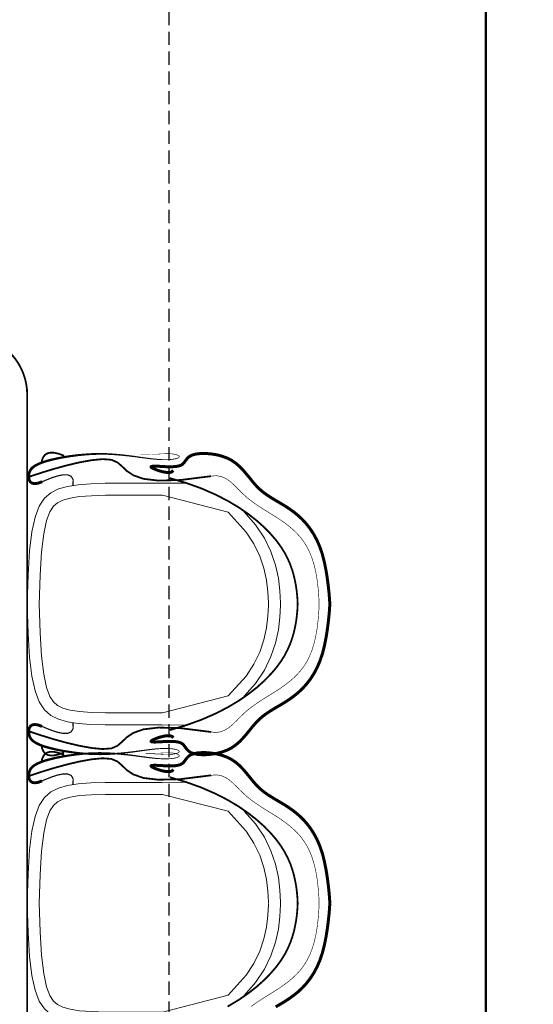
# Model space of a CAD drawing. Units: inches. Extents: x 513 to 1142, y 396 to 927.
# Tile 18 of 31: x 818 to 838, y 728 to 766. Entities that reach past the tile are written whole.
import ezdxf

# ---------------------------------------------------------------- set-up
doc = ezdxf.new("R2010")
doc.units = ezdxf.units.IN
doc.header["$MEASUREMENT"] = 0
doc.linetypes.add('DASHED', pattern=[0.75, 0.5, -0.25])
for name, color, linetype, lineweight in [('A-ANNO-DIMS', 2, 'DASHED', 18), ('A-WALL', 7, 'Continuous', 50), ('furniture', 92, 'Continuous', 18)]:
    doc.layers.add(name, color=color, linetype=linetype, lineweight=lineweight)
doc.styles.get("Standard").update_dxf_attribs({"font": 'arial.ttf'})
doc.dimstyles.get("Standard").update_dxf_attribs({"dimtxt": 4, "dimasz": 0.18, "dimexe": 0.18, "dimexo": 0.0625, "dimgap": 0.09, "dimtad": 0, "dimtih": 1, "dimtoh": 1, "dimdec": 0, "dimrnd": 6, "dimzin": 0, "dimdsep": 46, "dimlunit": 3, "dimtxsty": 'Standard', "dimcen": 0.09, "dimadec": 0, "dimazin": 0, "dimtfac": 1, "dimtdec": 0, "dimtofl": 0, "dimtmove": 0, "dimatfit": 3, "dimfxl": 1, "dimtolj": 1, "dimtzin": 0, "dimarcsym": 0})

# ---------------------------------------------------------------- blocks, each defined once
blk = doc.blocks.new('ОГ55_на6персон_стол1400х900')
at = {"const_width": 3}
blk.add_lwpolyline([(-600, 279.3), (600, 279.3, -0.414214), (700, 179.3), (700, -520.7, -0.414214), (600, -620.7), (-600, -620.7, -0.414214), (-700, -520.7), (-700, 179.3, -0.414214)], format="xyb", close=True, dxfattribs=at)
for points in [[(-452.3, -886.8), (-451.9, -846.4), (-451.9, -810.6), (-452, -778.9), (-451.9, -751.1), (-451.2, -726.9), (-449.6, -706), (-446.8, -688.1), (-442.5, -672.9), (-436.1, -660), (-426.8, -649.4), (-413.5, -640.7), (-395.1, -633.9), (-370.6, -628.7), (-339, -624.8), (-299.1, -622.2), (-250, -620.7)], [(-47.7, -886.8), (-48.1, -846.4), (-48.1, -810.6), (-48, -778.9), (-48.1, -751.1), (-48.8, -726.9), (-50.4, -706), (-53.2, -688.1), (-57.5, -672.9), (-63.9, -660), (-73.2, -649.4), (-86.5, -640.7), (-104.9, -633.9), (-129.4, -628.7), (-161, -624.8), (-200.9, -622.2), (-250, -620.7)], [(47.7, -886.8), (48.1, -846.4), (48.1, -810.6), (48, -778.9), (48.1, -751.1), (48.8, -726.9), (50.4, -706), (53.2, -688.1), (57.5, -672.9), (63.9, -660), (73.2, -649.4), (86.5, -640.7), (104.9, -633.9), (129.4, -628.7), (161, -624.8), (200.9, -622.2), (250, -620.7)], [(452.3, -886.8), (451.9, -846.4), (451.9, -810.6), (452, -778.9), (451.9, -751.1), (451.2, -726.9), (449.6, -706), (446.8, -688.1), (442.5, -672.9), (436.1, -660), (426.8, -649.4), (413.5, -640.7), (395.1, -633.9), (370.6, -628.7), (339, -624.8), (299.1, -622.2), (250, -620.7)], [(-403.6, -956.4), (-431.9, -846.6), (-431.9, -810.5), (-432, -778.9), (-431.9, -751.4), (-431.2, -728), (-429.8, -708.3), (-427.3, -692.4), (-423.8, -680.1), (-419.4, -671.3), (-413.6, -664.7), (-404.4, -658.7), (-389.5, -653.1), (-367.3, -648.4), (-337.1, -644.8), (-298.1, -642.2), (-249.4, -640.7)], [(-96.4, -956.4), (-68.1, -846.6), (-68.1, -810.5), (-68, -778.9), (-68.1, -751.4), (-68.8, -728), (-70.2, -708.3), (-72.7, -692.4), (-76.2, -680.1), (-80.6, -671.3), (-86.4, -664.7), (-95.6, -658.7), (-110.5, -653.1), (-132.7, -648.4), (-162.9, -644.8), (-201.9, -642.2), (-250.6, -640.7)], [(96.4, -956.4), (68.1, -846.6), (68.1, -810.5), (68, -778.9), (68.1, -751.4), (68.8, -728), (70.2, -708.3), (72.7, -692.4), (76.2, -680.1), (80.6, -671.3), (86.4, -664.7), (95.6, -658.7), (110.5, -653.1), (132.7, -648.4), (162.9, -644.8), (201.9, -642.2), (250.6, -640.7)], [(403.6, -956.4), (431.9, -846.6), (431.9, -810.5), (432, -778.9), (431.9, -751.4), (431.2, -728), (429.8, -708.3), (427.3, -692.4), (423.8, -680.1), (419.4, -671.3), (413.6, -664.7), (404.4, -658.7), (389.5, -653.1), (367.3, -648.4), (337.1, -644.8), (298.1, -642.2), (249.4, -640.7)], [(-403.6, -956.4), (-370.3, -986.3), (-350.5, -999.5), (-330.2, -1009.3), (-309.8, -1016.2), (-289.8, -1020.6), (-270.4, -1023), (-252.1, -1023.8), (-250.4, -1023.8)], [(-96.4, -956.4), (-129.7, -986.3), (-149.5, -999.5), (-169.8, -1009.3), (-190.2, -1016.2), (-210.2, -1020.6), (-229.6, -1023), (-247.9, -1023.8), (-249.6, -1023.8)], [(96.4, -956.4), (129.7, -986.3), (149.5, -999.5), (169.8, -1009.3), (190.2, -1016.2), (210.2, -1020.6), (229.6, -1023), (247.9, -1023.8), (249.6, -1023.8)], [(403.6, -956.4), (370.3, -986.3), (350.5, -999.5), (330.2, -1009.3), (309.8, -1016.2), (289.8, -1020.6), (270.4, -1023), (252.1, -1023.8), (250.4, -1023.8)], [(-404, -983), (-382.6, -1002.1), (-360.4, -1016.9), (-337.8, -1027.9), (-315.2, -1035.5), (-293.1, -1040.4), (-272, -1043), (-252.3, -1043.8), (-250, -1043.8)], [(-96, -983), (-117.4, -1002.1), (-139.6, -1016.9), (-162.2, -1027.9), (-184.8, -1035.5), (-206.9, -1040.4), (-228, -1043), (-247.7, -1043.8), (-250, -1043.8)], [(96, -983), (117.4, -1002.1), (139.6, -1016.9), (162.2, -1027.9), (184.8, -1035.5), (206.9, -1040.4), (228, -1043), (247.7, -1043.8), (250, -1043.8)], [(404, -983), (382.6, -1002.1), (360.4, -1016.9), (337.8, -1027.9), (315.2, -1035.5), (293.1, -1040.4), (272, -1043), (252.3, -1043.8), (250, -1043.8)]]:
    blk.add_lwpolyline(points)
for points in [[(-45.5, -645.6, 5, 4.91, 0), (-48, -638.8, 4.91, 4.84, 0), (-48.7, -633.5, 4.84, 4.78, 0), (-48.1, -629.4, 4.78, 4.74, 0), (-46.3, -626.5, 4.74, 4.7, 0), (-43.7, -624.6, 4.7, 4.65, 0), (-40.6, -623.5, 4.65, 4.61, 0), (-37.1, -623.2, 4.61, 4.56, 0), (-33.5, -623.5, 4.56, 4.52, 0), (-30.2, -624.2, 4.52, 4.47, 0), (-27.1, -625.5, 4.47, 4.43, 0), (-24.1, -627.4, 4.43, 4.38, 0), (-21.3, -630.2, 4.38, 4.32, 0), (-18.7, -633.9, 4.32, 4.25, 0), (-16.2, -638.6, 4.25, 4.17, 0), (-13.7, -644.5, 4.17, 4.07, 0), (-11.3, -651.7, 4.07, 3.95, 0), (-9, -660.3, 3.95, 3.82, 0), (-6.7, -670, 3.82, 3.68, 0), (-4.6, -680.8, 3.68, 3.53, 0), (-2.8, -692.3, 3.53, 3.37, 0), (-1.2, -704.4, 3.37, 3.21, 0), (0, -716.9, 3.21, 3.05, 0), (0.8, -729.5, 3.05, 2.88, 0), (1.1, -742.1, 2.88, 2.72, 0), (0.9, -754.5, 2.72, 2.57, 0), (0.2, -766.5, 2.57, 2.41, 0), (-0.8, -778.1, 2.41, 2.27, 0), (-2, -789.2, 2.27, 2.13, 0), (-3.3, -799.7, 2.13, 2, 0), (-4.7, -809.6, 2, 1.88, 0), (-5.9, -818.7, 1.88, 1.78, 0), (-7, -827, 1.78, 1.68, 0), (-7.8, -834.4, 1.68, 1.59, 0), (-8.3, -841, 1.59, 1.52, 0), (-8.6, -846.8, 1.52, 1.45, 0), (-8.7, -851.9, 1.45, 1.4, 0), (-8.6, -856.3, 1.4, 1.35, 0), (-8.4, -860.1, 1.35, 1.3, 0), (-8, -863.3, 1.3, 1.27, 0), (-7.6, -866, 1.27, 1.24, 0), (-7.2, -868.3, 1.24, 1.21, 0), (-6.7, -870.2, 1.21, 1.19, 0), (-6.2, -871.7, 1.19, 1.18, 0), (-5.7, -872.9, 1.18, 1.16, 0), (-5.2, -873.7, 1.16, 1.15, 0), (-4.7, -874.3, 1.15, 1.14, 0), (-4.2, -874.6, 1.14, 1.14, 0), (-3.7, -874.7, 1.14, 1.13, 0), (-3.2, -874.6, 1.13, 1.12, 0), (-2.7, -874.3, 1.12, 1.12, 0), (-2.2, -873.9, 1.12, 1.11, 0), (-1.7, -873.3, 1.11, 1.09, 0), (-1.3, -872.5, 1.09, 1.08, 0), (-0.9, -871.6, 1.08, 1.07, 0), (-0.5, -870.5, 1.07, 1.05, 0), (-0.1, -869.2, 1.05, 1.03, 0), (0.3, -867.9, 1.03, 1.01, 0), (0.6, -866.3, 1.01, 0.986, 0), (0.9, -864.5, 0.986, 0.959, 0), (1.1, -862.4, 0.959, 0.926, 0), (1.3, -859.9, 0.926, 0.889, 0), (1.4, -857, 0.889, 0.846, 0), (1.4, -853.7, 0.846, 0.796, 0), (1.3, -849.8, 0.796, 0.738, 0), (1.1, -845.4, 0.738, 0.672, 0), (0.8, -840.3, 0.672, 0.595, 0), (0.6, -834.3, 0.595, 0.506, 0), (0.3, -827.5, 0.506, 0.404, 0), (0.1, -819.6, 0.404, 0.286, 0), (-0.1, -810.5, 0.286, 0.152, 0), (-0.1, -800.2, 0.152, 0, 0), (0, -788.5, 0, 0, 0)], [(45.5, -645.6, 5, 4.91, 0), (48, -638.8, 4.91, 4.84, 0), (48.7, -633.5, 4.84, 4.78, 0), (48.1, -629.4, 4.78, 4.74, 0), (46.3, -626.5, 4.74, 4.7, 0), (43.7, -624.6, 4.7, 4.65, 0), (40.6, -623.5, 4.65, 4.61, 0), (37.1, -623.2, 4.61, 4.56, 0), (33.5, -623.5, 4.56, 4.52, 0), (30.2, -624.2, 4.52, 4.47, 0), (27.1, -625.5, 4.47, 4.43, 0), (24.1, -627.4, 4.43, 4.38, 0), (21.3, -630.2, 4.38, 4.32, 0), (18.7, -633.9, 4.32, 4.25, 0), (16.2, -638.6, 4.25, 4.17, 0), (13.7, -644.5, 4.17, 4.07, 0), (11.3, -651.7, 4.07, 3.95, 0), (9, -660.3, 3.95, 3.82, 0), (6.7, -670, 3.82, 3.68, 0), (4.6, -680.8, 3.68, 3.53, 0), (2.8, -692.3, 3.53, 3.37, 0), (1.2, -704.4, 3.37, 3.21, 0), (0, -716.9, 3.21, 3.05, 0), (-0.8, -729.5, 3.05, 2.88, 0), (-1.1, -742.1, 2.88, 2.72, 0), (-0.9, -754.5, 2.72, 2.57, 0), (-0.2, -766.5, 2.57, 2.41, 0), (0.8, -778.1, 2.41, 2.27, 0), (2, -789.2, 2.27, 2.13, 0), (3.3, -799.7, 2.13, 2, 0), (4.7, -809.6, 2, 1.88, 0), (5.9, -818.7, 1.88, 1.78, 0), (7, -827, 1.78, 1.68, 0), (7.8, -834.4, 1.68, 1.59, 0), (8.3, -841, 1.59, 1.52, 0), (8.6, -846.8, 1.52, 1.45, 0), (8.7, -851.9, 1.45, 1.4, 0), (8.6, -856.3, 1.4, 1.35, 0), (8.4, -860.1, 1.35, 1.3, 0), (8, -863.3, 1.3, 1.27, 0), (7.6, -866, 1.27, 1.24, 0), (7.2, -868.3, 1.24, 1.21, 0), (6.7, -870.2, 1.21, 1.19, 0), (6.2, -871.7, 1.19, 1.18, 0), (5.7, -872.9, 1.18, 1.16, 0), (5.2, -873.7, 1.16, 1.15, 0), (4.7, -874.3, 1.15, 1.14, 0), (4.2, -874.6, 1.14, 1.14, 0), (3.7, -874.7, 1.14, 1.13, 0), (3.2, -874.6, 1.13, 1.12, 0), (2.7, -874.3, 1.12, 1.12, 0), (2.2, -873.9, 1.12, 1.11, 0), (1.7, -873.3, 1.11, 1.09, 0), (1.3, -872.5, 1.09, 1.08, 0), (0.9, -871.6, 1.08, 1.07, 0), (0.5, -870.5, 1.07, 1.05, 0), (0.1, -869.2, 1.05, 1.03, 0), (-0.3, -867.9, 1.03, 1.01, 0), (-0.6, -866.3, 1.01, 0.986, 0), (-0.9, -864.5, 0.986, 0.959, 0), (-1.1, -862.4, 0.959, 0.926, 0), (-1.3, -859.9, 0.926, 0.889, 0), (-1.4, -857, 0.889, 0.846, 0), (-1.4, -853.7, 0.846, 0.796, 0), (-1.3, -849.8, 0.796, 0.738, 0), (-1.1, -845.4, 0.738, 0.672, 0), (-0.8, -840.3, 0.672, 0.595, 0), (-0.6, -834.3, 0.595, 0.506, 0), (-0.3, -827.5, 0.506, 0.404, 0), (-0.1, -819.6, 0.404, 0.286, 0), (0.1, -810.5, 0.286, 0.152, 0), (0.1, -800.2, 0.152, 0, 0), (0, -788.5, 0, 0, 0)], [(454.5, -645.6, 5, 4.91, 0), (452, -638.8, 4.91, 4.84, 0), (451.3, -633.5, 4.84, 4.78, 0), (451.9, -629.4, 4.78, 4.74, 0), (453.7, -626.5, 4.74, 4.7, 0), (456.3, -624.6, 4.7, 4.65, 0), (459.4, -623.5, 4.65, 4.61, 0), (462.9, -623.2, 4.61, 4.56, 0), (466.5, -623.5, 4.56, 4.52, 0), (469.8, -624.2, 4.52, 4.47, 0), (472.9, -625.5, 4.47, 4.43, 0), (475.9, -627.4, 4.43, 4.38, 0), (478.7, -630.2, 4.38, 4.32, 0), (481.3, -633.9, 4.32, 4.25, 0), (483.8, -638.6, 4.25, 4.17, 0), (486.3, -644.5, 4.17, 4.07, 0), (488.7, -651.7, 4.07, 3.95, 0), (491, -660.3, 3.95, 3.82, 0), (493.3, -670, 3.82, 3.68, 0), (495.4, -680.8, 3.68, 3.53, 0), (497.2, -692.3, 3.53, 3.37, 0), (498.8, -704.4, 3.37, 3.21, 0), (500, -716.9, 3.21, 3.05, 0), (500.8, -729.5, 3.05, 2.88, 0), (501.1, -742.1, 2.88, 2.72, 0), (500.9, -754.5, 2.72, 2.57, 0), (500.2, -766.5, 2.57, 2.41, 0), (499.2, -778.1, 2.41, 2.27, 0), (498, -789.2, 2.27, 2.13, 0), (496.7, -799.7, 2.13, 2, 0), (495.3, -809.6, 2, 1.88, 0), (494.1, -818.7, 1.88, 1.78, 0), (493, -827, 1.78, 1.68, 0), (492.2, -834.4, 1.68, 1.59, 0), (491.7, -841, 1.59, 1.52, 0), (491.4, -846.8, 1.52, 1.45, 0), (491.3, -851.9, 1.45, 1.4, 0), (491.4, -856.3, 1.4, 1.35, 0), (491.6, -860.1, 1.35, 1.3, 0), (492, -863.3, 1.3, 1.27, 0), (492.4, -866, 1.27, 1.24, 0), (492.8, -868.3, 1.24, 1.21, 0), (493.3, -870.2, 1.21, 1.19, 0), (493.8, -871.7, 1.19, 1.18, 0), (494.3, -872.9, 1.18, 1.16, 0), (494.8, -873.7, 1.16, 1.15, 0), (495.3, -874.3, 1.15, 1.14, 0), (495.8, -874.6, 1.14, 1.14, 0), (496.3, -874.7, 1.14, 1.13, 0), (496.8, -874.6, 1.13, 1.12, 0), (497.3, -874.3, 1.12, 1.12, 0), (497.8, -873.9, 1.12, 1.11, 0), (498.3, -873.3, 1.11, 1.09, 0), (498.7, -872.5, 1.09, 1.08, 0), (499.1, -871.6, 1.08, 1.07, 0), (499.5, -870.5, 1.07, 1.05, 0), (499.9, -869.2, 1.05, 1.03, 0), (500.3, -867.9, 1.03, 1.01, 0), (500.6, -866.3, 1.01, 0.986, 0), (500.9, -864.5, 0.986, 0.959, 0), (501.1, -862.4, 0.959, 0.926, 0), (501.3, -859.9, 0.926, 0.889, 0), (501.4, -857, 0.889, 0.846, 0), (501.4, -853.7, 0.846, 0.796, 0), (501.3, -849.8, 0.796, 0.738, 0), (501.1, -845.4, 0.738, 0.672, 0), (500.8, -840.3, 0.672, 0.595, 0), (500.6, -834.3, 0.595, 0.506, 0), (500.3, -827.5, 0.506, 0.404, 0), (500.1, -819.6, 0.404, 0.286, 0), (499.9, -810.5, 0.286, 0.152, 0), (499.9, -800.2, 0.152, 0, 0), (500, -788.5, 0, 0, 0)]]:
    blk.add_lwpolyline(points, format="xyseb")
for points, const_width in [([(-36.2, -927.9), (-42.6, -876.9), (-43.6, -840.1), (-40.6, -814.7), (-34.7, -798), (-27.4, -787), (-19.8, -779.2), (-13.2, -771.5), (-8.8, -761.4), (-7.7, -746.6), (-9.5, -728.1), (-13.3, -707.3), (-18.4, -685.8), (-24.1, -665.1), (-29.7, -646.8), (-34.4, -632.3), (-37.5, -623.2)], 3), ([(36.2, -927.9), (42.6, -876.9), (43.6, -840.1), (40.6, -814.7), (34.7, -798), (27.4, -787), (19.8, -779.2), (13.2, -771.5), (8.8, -761.4), (7.7, -746.6), (9.5, -728.1), (13.3, -707.3), (18.4, -685.8), (24.1, -665.1), (29.7, -646.8), (34.4, -632.3), (37.5, -623.2)], 3), ([(463.8, -927.9), (457.4, -876.9), (456.4, -840.1), (459.4, -814.7), (465.3, -798), (472.6, -787), (480.2, -779.2), (486.8, -771.5), (491.2, -761.4), (492.3, -746.6), (490.5, -728.1), (486.7, -707.3), (481.6, -685.8), (475.9, -665.1), (470.3, -646.8), (465.6, -632.3), (462.5, -623.2)], 3), ([(-45.5, -645.6), (-42.2, -653.4), (-38.7, -662.3), (-35.7, -671.7), (-33.9, -680.7), (-34, -688.5), (-36.5, -694.3), (-42.2, -697.5), (-51.8, -697.1)], 2), ([(-2, -682.4), (1.3, -673.2), (3, -665.5), (3.1, -659.2), (1.9, -654.2), (-0.6, -650.4), (-4.2, -647.6), (-8.8, -645.6), (-14.3, -644.5)], 3), ([(2, -682.4), (-1.3, -673.2), (-3, -665.5), (-3.1, -659.2), (-1.9, -654.2), (0.6, -650.4), (4.2, -647.6), (8.8, -645.6), (14.3, -644.5)], 3), ([(45.5, -645.6), (42.2, -653.4), (38.7, -662.3), (35.7, -671.7), (33.9, -680.7), (34, -688.5), (36.5, -694.3), (42.2, -697.5), (51.8, -697.1)], 2), ([(454.5, -645.6), (457.8, -653.4), (461.3, -662.3), (464.3, -671.7), (466.1, -680.7), (466, -688.5), (463.5, -694.3), (457.8, -697.5), (448.2, -697.1)], 2), ([(498, -682.4), (501.3, -673.2), (503, -665.5), (503.1, -659.2), (501.9, -654.2), (499.4, -650.4), (495.8, -647.6), (491.2, -645.6), (485.7, -644.5)], 3), ([(-423.2, -1035.9), (-418.9, -1043.3), (-414.4, -1050.8), (-409.5, -1058.3), (-404.2, -1065.7), (-398.3, -1073), (-391.7, -1080.1), (-384.3, -1086.9), (-376.1, -1093.3), (-366.9, -1099.3), (-356.7, -1104.8), (-345.4, -1109.7), (-333, -1113.9), (-319.5, -1117.3), (-305.4, -1120.1), (-291.5, -1122.3), (-278.6, -1123.9), (-267.2, -1125.1), (-258.2, -1125.8), (-252.2, -1126.2), (-250, -1126.3)], 5), ([(-26.6, -864.8), (-28.8, -862.7), (-29.9, -859.6), (-30.1, -855.5), (-29.6, -851), (-28.6, -846.2), (-27.3, -841.5), (-25.8, -837.1), (-24.3, -833.4), (-23, -830.6), (-22, -828.7), (-21.1, -827.8), (-20.4, -827.7), (-19.9, -828.6), (-19.6, -830.5), (-19.4, -833.2), (-19.5, -836.7), (-19.7, -841.2), (-20, -846.2), (-20.3, -851.7), (-20.4, -857.3), (-20.4, -862.9), (-20.1, -868.2), (-19.4, -872.9), (-18.2, -876.8), (-16.5, -879.9), (-14.3, -882.2), (-11.8, -884.1), (-9.2, -886), (-6.6, -888), (-4.1, -890.6), (-1.9, -894), (-0.2, -898.6), (1.1, -904.5), (1.7, -911.6), (1.7, -919.5), (1, -928), (-0.4, -936.8), (-2.6, -945.6), (-5.7, -954.1), (-9.6, -962), (-14.5, -969.1), (-20, -975.5), (-26.1, -981.4), (-32.5, -986.9), (-39.1, -992.3), (-45.7, -997.6), (-51.9, -1003), (-57.8, -1008.8), (-63.1, -1015.1), (-67.9, -1021.7), (-72.4, -1028.7), (-76.8, -1035.9), (-81.1, -1043.3), (-85.6, -1050.8), (-90.5, -1058.3), (-95.8, -1065.7), (-101.7, -1073), (-108.3, -1080.1), (-115.7, -1086.9), (-123.9, -1093.3), (-133.1, -1099.3), (-143.3, -1104.8), (-154.6, -1109.7), (-167, -1113.9), (-180.5, -1117.3), (-194.6, -1120.1), (-208.5, -1122.3), (-221.4, -1123.9), (-232.8, -1125.1), (-241.8, -1125.8), (-247.8, -1126.2), (-250, -1126.3)], 5), ([(26.6, -864.8), (28.8, -862.7), (29.9, -859.6), (30.1, -855.5), (29.6, -851), (28.6, -846.2), (27.3, -841.5), (25.8, -837.1), (24.3, -833.4), (23, -830.6), (22, -828.7), (21.1, -827.8), (20.4, -827.7), (19.9, -828.6), (19.6, -830.5), (19.4, -833.2), (19.5, -836.7), (19.7, -841.2), (20, -846.2), (20.3, -851.7), (20.4, -857.3), (20.4, -862.9), (20.1, -868.2), (19.4, -872.9), (18.2, -876.8), (16.5, -879.9), (14.3, -882.2), (11.8, -884.1), (9.2, -886), (6.6, -888), (4.1, -890.6), (1.9, -894), (0.2, -898.6), (-1.1, -904.5), (-1.7, -911.6), (-1.7, -919.5), (-1, -928), (0.4, -936.8), (2.6, -945.6), (5.7, -954.1), (9.6, -962), (14.5, -969.1), (20, -975.5), (26.1, -981.4), (32.5, -986.9), (39.1, -992.3), (45.7, -997.6), (51.9, -1003), (57.8, -1008.8), (63.1, -1015.1), (67.9, -1021.7), (72.4, -1028.7), (76.8, -1035.9), (81.1, -1043.3), (85.6, -1050.8), (90.5, -1058.3), (95.8, -1065.7), (101.7, -1073), (108.3, -1080.1), (115.7, -1086.9), (123.9, -1093.3), (133.1, -1099.3), (143.3, -1104.8), (154.6, -1109.7), (167, -1113.9), (180.5, -1117.3), (194.6, -1120.1), (208.5, -1122.3), (221.4, -1123.9), (232.8, -1125.1), (241.8, -1125.8), (247.8, -1126.2), (250, -1126.3)], 5), ([(473.4, -864.8), (471.2, -862.7), (470.1, -859.6), (469.9, -855.5), (470.4, -851), (471.4, -846.2), (472.7, -841.5), (474.2, -837.1), (475.7, -833.4), (477, -830.6), (478, -828.7), (478.9, -827.8), (479.6, -827.7), (480.1, -828.6), (480.4, -830.5), (480.6, -833.2), (480.5, -836.7), (480.3, -841.2), (480, -846.2), (479.7, -851.7), (479.6, -857.3), (479.6, -862.9), (479.9, -868.2), (480.6, -872.9), (481.8, -876.8), (483.5, -879.9), (485.7, -882.2), (488.2, -884.1), (490.8, -886), (493.4, -888), (495.9, -890.6), (498.1, -894), (499.8, -898.6), (501.1, -904.5), (501.7, -911.6), (501.7, -919.5), (501, -928), (499.6, -936.8), (497.4, -945.6), (494.3, -954.1), (490.4, -962), (485.5, -969.1), (480, -975.5), (473.9, -981.4), (467.5, -986.9), (460.9, -992.3), (454.3, -997.6), (448.1, -1003), (442.2, -1008.8), (436.9, -1015.1), (432.1, -1021.7), (427.6, -1028.7), (423.2, -1035.9), (418.9, -1043.3), (414.4, -1050.8), (409.5, -1058.3), (404.2, -1065.7), (398.3, -1073), (391.7, -1080.1), (384.3, -1086.9), (376.1, -1093.3), (366.9, -1099.3), (356.7, -1104.8), (345.4, -1109.7), (333, -1113.9), (319.5, -1117.3), (305.4, -1120.1), (291.5, -1122.3), (278.6, -1123.9), (267.2, -1125.1), (258.2, -1125.8), (252.2, -1126.2), (250, -1126.3)], 5), ([(-422.7, -955.5), (-411.8, -973.8), (-400.6, -990), (-389.4, -1004.3), (-378.2, -1016.8), (-367.2, -1027.5), (-356.5, -1036.7), (-346, -1044.4), (-335.8, -1050.8), (-325.7, -1056), (-315.9, -1060.3), (-306.4, -1063.6), (-297, -1066.3), (-287.9, -1068.3), (-279.3, -1069.9), (-271.3, -1071), (-264.3, -1071.7), (-258.4, -1072.2), (-253.9, -1072.4), (-251, -1072.5), (-250, -1072.5)], 3), ([(-39.4, -859), (-47.7, -886.8), (-56.8, -912.1), (-66.8, -934.9), (-77.3, -955.5), (-88.2, -973.8), (-99.4, -990), (-110.6, -1004.3), (-121.8, -1016.8), (-132.8, -1027.5), (-143.5, -1036.7), (-154, -1044.4), (-164.2, -1050.8), (-174.3, -1056), (-184.1, -1060.3), (-193.6, -1063.6), (-203, -1066.3), (-212.1, -1068.3), (-220.7, -1069.9), (-228.7, -1071), (-235.7, -1071.7), (-241.6, -1072.2), (-246.1, -1072.4), (-249, -1072.5), (-250, -1072.5)], 3), ([(39.4, -859), (47.7, -886.8), (56.8, -912.1), (66.8, -934.9), (77.3, -955.5), (88.2, -973.8), (99.4, -990), (110.6, -1004.3), (121.8, -1016.8), (132.8, -1027.5), (143.5, -1036.7), (154, -1044.4), (164.2, -1050.8), (174.3, -1056), (184.1, -1060.3), (193.6, -1063.6), (203, -1066.3), (212.1, -1068.3), (220.7, -1069.9), (228.7, -1071), (235.7, -1071.7), (241.6, -1072.2), (246.1, -1072.4), (249, -1072.5), (250, -1072.5)], 3), ([(460.6, -859), (452.3, -886.8), (443.2, -912.1), (433.2, -934.9), (422.7, -955.5), (411.8, -973.8), (400.6, -990), (389.4, -1004.3), (378.2, -1016.8), (367.2, -1027.5), (356.5, -1036.7), (346, -1044.4), (335.8, -1050.8), (325.7, -1056), (315.9, -1060.3), (306.4, -1063.6), (297, -1066.3), (287.9, -1068.3), (279.3, -1069.9), (271.3, -1071), (264.3, -1071.7), (258.4, -1072.2), (253.9, -1072.4), (251, -1072.5), (250, -1072.5)], 3), ([(-422.8, -994.6), (-417.9, -1001.3), (-413.3, -1008.1), (-408.8, -1015), (-404.4, -1022.1), (-400, -1029.2), (-395.5, -1036.4), (-390.8, -1043.6), (-385.8, -1050.7), (-380.5, -1057.7), (-374.7, -1064.5), (-368.5, -1071), (-361.7, -1077.1), (-354.1, -1082.8), (-345.9, -1088), (-336.7, -1092.6), (-326.7, -1096.6), (-315.5, -1100), (-303.3, -1102.9), (-289.8, -1105.2), (-274.9, -1106.9), (-258.6, -1108.1), (-250, -1108.4)], 1), ([(-36.2, -927.9), (-35.4, -936.5), (-36.6, -944.3), (-39.5, -951.4), (-43.7, -958), (-48.9, -964.1), (-54.7, -970.1), (-60.7, -976), (-66.6, -982), (-72.1, -988.2), (-77.2, -994.6), (-82.1, -1001.3), (-86.7, -1008.1), (-91.2, -1015), (-95.6, -1022.1), (-100, -1029.2), (-104.5, -1036.4), (-109.2, -1043.6), (-114.2, -1050.7), (-119.5, -1057.7), (-125.3, -1064.5), (-131.5, -1071), (-138.3, -1077.1), (-145.9, -1082.8), (-154.1, -1088), (-163.3, -1092.6), (-173.3, -1096.6), (-184.5, -1100), (-196.7, -1102.9), (-210.2, -1105.2), (-225.1, -1106.9), (-241.4, -1108.1), (-250, -1108.4)], 1), ([(36.2, -927.9), (35.4, -936.5), (36.6, -944.3), (39.5, -951.4), (43.7, -958), (48.9, -964.1), (54.7, -970.1), (60.7, -976), (66.6, -982), (72.1, -988.2), (77.2, -994.6), (82.1, -1001.3), (86.7, -1008.1), (91.2, -1015), (95.6, -1022.1), (100, -1029.2), (104.5, -1036.4), (109.2, -1043.6), (114.2, -1050.7), (119.5, -1057.7), (125.3, -1064.5), (131.5, -1071), (138.3, -1077.1), (145.9, -1082.8), (154.1, -1088), (163.3, -1092.6), (173.3, -1096.6), (184.5, -1100), (196.7, -1102.9), (210.2, -1105.2), (225.1, -1106.9), (241.4, -1108.1), (250, -1108.4)], 1), ([(463.8, -927.9), (464.6, -936.5), (463.4, -944.3), (460.5, -951.4), (456.3, -958), (451.1, -964.1), (445.3, -970.1), (439.3, -976), (433.4, -982), (427.9, -988.2), (422.8, -994.6), (417.9, -1001.3), (413.3, -1008.1), (408.8, -1015), (404.4, -1022.1), (400, -1029.2), (395.5, -1036.4), (390.8, -1043.6), (385.8, -1050.7), (380.5, -1057.7), (374.7, -1064.5), (368.5, -1071), (361.7, -1077.1), (354.1, -1082.8), (345.9, -1088), (336.7, -1092.6), (326.7, -1096.6), (315.5, -1100), (303.3, -1102.9), (289.8, -1105.2), (274.9, -1106.9), (258.6, -1108.1), (250, -1108.4)], 1)]:
    blk.add_lwpolyline(points, dxfattribs=dict(const_width=const_width))
blk = doc.blocks.new('*D136')
at = {"layer": 'A-ANNO-DIMS', "color": 0, "lineweight": -2, "transparency": 16777216}
for p, q in [((835.995, 770.096), (835.995, 401.578)), ((743.802, 768.607), (743.802, 401.578)), ((743.982, 401.758), (784.509, 401.758)), ((835.815, 401.758), (795.289, 401.758))]:
    blk.add_line(p, q, dxfattribs=at)
at = {"layer": 'A-ANNO-DIMS', "color": 0, "transparency": 16777216}
for points in [[(743.982, 401.788), (743.982, 401.728), (743.802, 401.758)], [(835.815, 401.788), (835.815, 401.728), (835.995, 401.758)]]:
    blk.add_solid(points, dxfattribs=at)
at = {"layer": 'Defpoints', "color": 0, "transparency": 16777216}
for p in [(835.995, 770.158), (743.802, 768.67), (835.995, 401.758)]:
    blk.add_point(p, dxfattribs=at)
at = {"layer": 'A-ANNO-DIMS', "color": 0, "transparency": 16777216, "insert": (789.899, 401.758), "char_height": 4, "attachment_point": 5}
blk.add_mtext('\\A1;7\'-8"', dxfattribs=at)
blk = doc.blocks.new('*D169')
at = {"layer": 'A-ANNO-DIMS', "color": 0, "lineweight": -2, "transparency": 16777216}
for p, q in [((835.995, 774.096), (835.995, 401.578)), ((839.995, 774.096), (839.995, 401.578)), ((836.175, 401.758), (839.815, 401.758)), ((839.995, 401.758), (840.175, 401.758))]:
    blk.add_line(p, q, dxfattribs=at)
at = {"layer": 'A-ANNO-DIMS', "color": 0, "transparency": 16777216}
for points in [[(836.175, 401.788), (836.175, 401.728), (835.995, 401.758)], [(839.815, 401.788), (839.815, 401.728), (839.995, 401.758)]]:
    blk.add_solid(points, dxfattribs=at)
at = {"layer": 'Defpoints', "color": 0, "transparency": 16777216}
for p in [(835.995, 774.158), (839.995, 774.158), (839.995, 401.758)]:
    blk.add_point(p, dxfattribs=at)
at = {"layer": 'A-ANNO-DIMS', "color": 0, "transparency": 16777216, "insert": (845.582, 401.758), "char_height": 4, "attachment_point": 5}
blk.add_mtext('\\A1;0\'-4"', dxfattribs=at)
blk = doc.blocks.new('*D175')
at = {"layer": 'A-ANNO-DIMS', "color": 0, "lineweight": -2, "transparency": 16777216}
for p, q in [((772.995, 637.221), (772.995, 920.738)), ((823.995, 637.221), (823.995, 920.738)), ((773.175, 920.558), (793.008, 920.558)), ((823.815, 920.558), (803.982, 920.558))]:
    blk.add_line(p, q, dxfattribs=at)
at = {"layer": 'A-ANNO-DIMS', "color": 0, "transparency": 16777216}
for points in [[(773.175, 920.588), (773.175, 920.528), (772.995, 920.558)], [(823.815, 920.588), (823.815, 920.528), (823.995, 920.558)]]:
    blk.add_solid(points, dxfattribs=at)
at = {"layer": 'Defpoints', "color": 0, "transparency": 16777216}
for p in [(823.995, 920.558), (772.995, 637.158), (823.995, 637.158)]:
    blk.add_point(p, dxfattribs=at)
at = {"layer": 'A-ANNO-DIMS', "color": 0, "transparency": 16777216, "insert": (798.495, 920.558), "char_height": 4, "attachment_point": 5}
blk.add_mtext('\\A1;4\'-3"', dxfattribs=at)

msp = doc.modelspace()

# ---------------------------------------------------------------- linework, layer by layer
at = {"layer": 'A-WALL'}
msp.add_line((835.995, 770.158), (835.995, 641.158), dxfattribs=at)

# ---------------------------------------------------------------- block references
at = {"layer": 'furniture', "xscale": 0.022676467704094, "yscale": 0.022676467704094, "zscale": 0.022676467704094, "rotation": 90}
msp.add_blockref('ОГ55_на6персон_стол1400х900', (804.54, 737.859), dxfattribs=at)

# ---------------------------------------------------------------- dimensions: what is measured, and where the dimension line sits
at = {"layer": 'A-ANNO-DIMS'}
for base, p1, p2, picture, middle in [((823.995, 920.558), (772.995, 637.158), (823.995, 637.158), '*D175', (798.495, 920.558)), ((839.995, 401.758), (835.995, 774.158), (839.995, 774.158), '*D169', (845.582, 401.758)), ((835.995, 401.758), (743.802, 768.67), (835.995, 770.158), '*D136', (789.899, 401.758))]:
    dim = msp.add_linear_dim(base=base, p1=p1, p2=p2, dimstyle='Standard', override={"dimdec": 1, "dimlfac": 1, "dimrnd": 0, "dimzin": 1, "dimdsep": 46, "dimlunit": 4, "dimfrac": 2}, dxfattribs=at)
    dim.commit()
    dim.dimension.update_dxf_attribs({"geometry": picture, "text_midpoint": middle})

doc.saveas('drawing.dxf')
